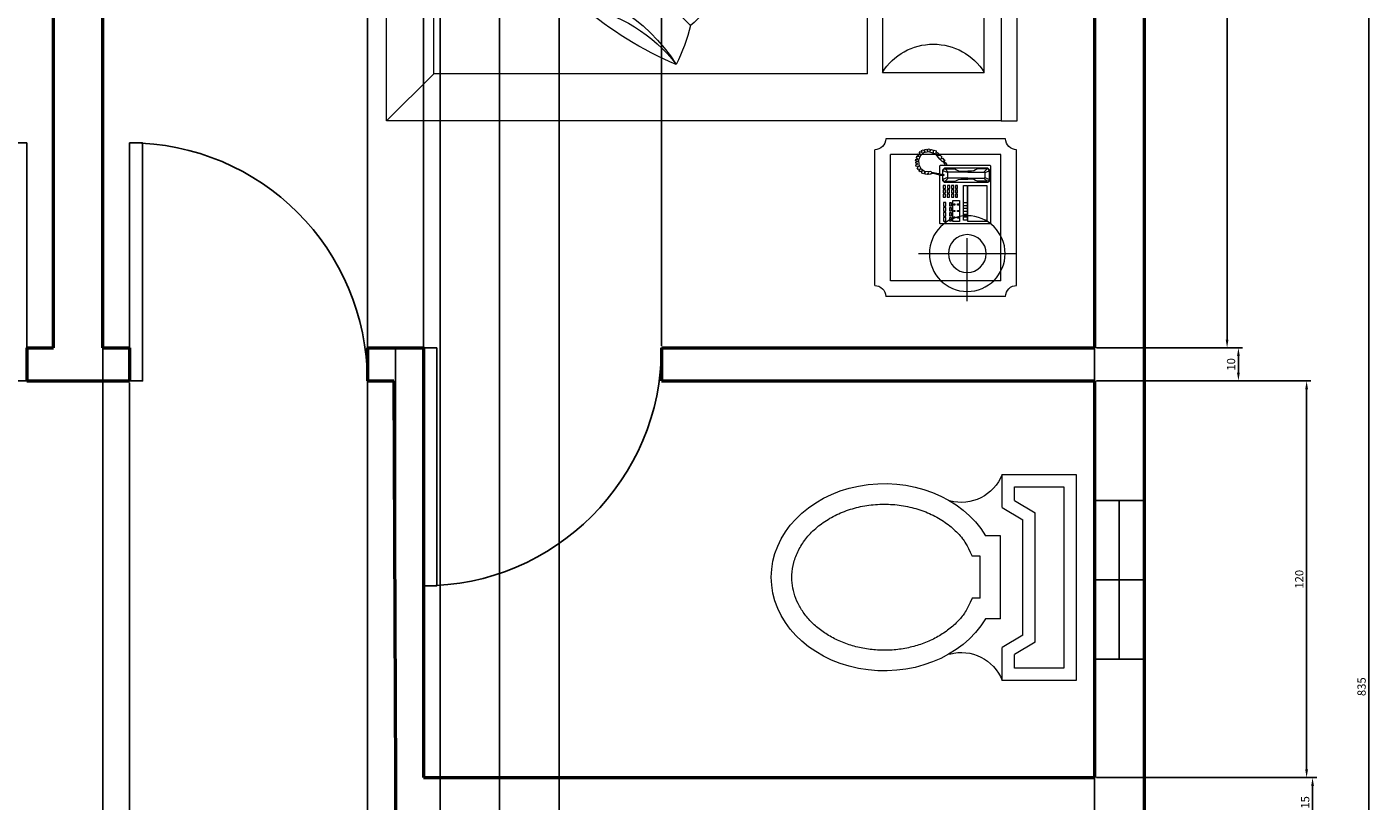
# Model space of a CAD drawing. Units: inches. Extents: x 604 to 3492, y -123 to 1737.
# Tile 16 of 20: x 1912 to 2319, y 836 to 1070. Entities that reach past the tile are written whole.
import ezdxf

# ---------------------------------------------------------------- set-up
doc = ezdxf.new("R2010")
doc.units = ezdxf.units.IN
for name, color, linetype, lineweight in [('A-ANNO-DIMS', 2, 'Continuous', 18), ('A-DOOR', 3, 'Continuous', 25), ('A-FLOR-FIXT', 9, 'Continuous', 18), ('A-FURN', 8, 'Continuous', 18), ('A-GLAZ', 4, 'Continuous', 25), ('A-WALL', 7, 'Continuous', 50)]:
    doc.layers.add(name, color=color, linetype=linetype, lineweight=lineweight)
doc.styles.get("Standard").update_dxf_attribs({"font": 'arial.ttf'})
doc.dimstyles.new('ISO-25', dxfattribs={"dimtxt": 2.5, "dimasz": 2.5, "dimexe": 1.25, "dimexo": 0.625, "dimtad": 1, "dimtxsty": 'Standard', "dimcen": 2.5, "dimadec": 0, "dimazin": 0, "dimtfac": 1, "dimtmove": 0, "dimatfit": 3, "dimfxl": 1, "dimarcsym": 0})

# ---------------------------------------------------------------- blocks, each defined once
blk = doc.blocks.new('A$C50B66110')
for p, q in [((0.0503, 1.9981), (0.4803, 1.9981)), ((0.1513, 1.6871), (0.1513, 1.9967)), ((0.5716, 1.9488), (0.5716, 2)), ((0.5716, 2), (2.0719, 2)), ((2.0719, 1.9488), (2.0719, 2)), ((2.1051, 1.9643), (2.1051, 1.5843)), ((2.5701, 1.9993), (2.1401, 1.9993)), ((2.6051, 1.9643), (2.6051, 1.5843)), ((0.0153, 1.9631), (0.0153, 1.5831)), ((0.0653, 1.9481), (0.0653, 1.5981)), ((0.0653, 1.9481), (0.4653, 1.9481)), ((0.4653, 1.9481), (0.4653, 1.5981)), ((0.5153, 1.9631), (0.5153, 1.5831)), ((2.0719, 1.9488), (0.5716, 1.9488)), ((0.5716, 1.9488), (0.5716, 0)), ((2.0719, 0), (2.0719, 1.9488)), ((2.1551, 1.9493), (2.1551, 1.5993)), ((2.5551, 1.9493), (2.1551, 1.9493)), ((2.3505, 1.62), (2.3505, 1.9295)), ((2.5551, 1.9493), (2.5551, 1.5993)), ((0.7257, 1.5725), (0.7257, 1.8954)), ((0.7257, 1.8954), (1.2113, 1.8954)), ((1.2113, 1.8954), (1.2113, 1.5725)), ((1.4007, 1.5725), (1.4007, 1.8954)), ((1.4007, 1.8954), (1.8863, 1.8954)), ((1.8863, 1.8954), (1.8863, 1.5725)), ((0, 1.8416), (0.2001, 1.8416)), ((2.5018, 1.7744), (2.2017, 1.7744)), ((0.0653, 1.5981), (0.4653, 1.5981)), ((2.5551, 1.5993), (2.1551, 1.5993)), ((0.0503, 1.5481), (0.4803, 1.5481)), ((1.2113, 1.5725), (0.7257, 1.5725)), ((1.8863, 1.5725), (1.4007, 1.5725)), ((2.5701, 1.5493), (2.1401, 1.5493)), ((1.5665, 1.5254), (1.5665, 1.0802)), ((1.5665, 1.5254), (1.9219, 1.0802)), ((1.9219, 1.0802), (1.5665, 1.0802)), ((0.5716, 0), (0.7216, 0.15)), ((2.0719, 0), (1.9219, 0.15)), ((0.5716, 0), (2.0719, 0))]:
    blk.add_line(p, q)
at = {"linetype": 'ByBlock'}
for p, q in [((0.2481, 1.9162), (0.2458, 1.9139)), ((0.2458, 1.9139), (0.2458, 1.7562)), ((0.2481, 1.9162), (0.4287, 1.9162)), ((0.2526, 1.9036), (0.2526, 1.8431)), ((0.3669, 1.9036), (0.2526, 1.9036)), ((0.3669, 1.8431), (0.3669, 1.9036)), ((0.3772, 1.9071), (0.3818, 1.9128)), ((0.3772, 1.7688), (0.3772, 1.9071)), ((0.3818, 1.9094), (0.3807, 1.9048)), ((0.3807, 1.9048), (0.3807, 1.8739)), ((0.3807, 1.9048), (0.3909, 1.8945)), ((0.3818, 1.9128), (0.4161, 1.9128)), ((0.3864, 1.9116), (0.3818, 1.9094)), ((0.3921, 1.8968), (0.3864, 1.9116)), ((0.3864, 1.9116), (0.4138, 1.9116)), ((0.3909, 1.8945), (0.3921, 1.8968)), ((0.3909, 1.8431), (0.3909, 1.8945)), ((0.4081, 1.8968), (0.3921, 1.8968)), ((0.4081, 1.8968), (0.4138, 1.9116)), ((0.4092, 1.8945), (0.4081, 1.8968)), ((0.4195, 1.9048), (0.4092, 1.8945)), ((0.4092, 1.8431), (0.4092, 1.8945)), ((0.4138, 1.9116), (0.4184, 1.9094)), ((0.4161, 1.9128), (0.4218, 1.9071)), ((0.4184, 1.9094), (0.4195, 1.9048)), ((0.4195, 1.9048), (0.4195, 1.8739)), ((0.4218, 1.9071), (0.4218, 1.7699)), ((0.4287, 1.9162), (0.4309, 1.9139)), ((0.4309, 1.9139), (0.4309, 1.7562)), ((0.2526, 1.8431), (0.3669, 1.8431)), ((0.2572, 1.8408), (0.2572, 1.8294)), ((0.3669, 1.8408), (0.2572, 1.8408)), ((0.2664, 1.8408), (0.2664, 1.8294)), ((0.2755, 1.8408), (0.2755, 1.8294)), ((0.2846, 1.8408), (0.2846, 1.8294)), ((0.2938, 1.8408), (0.2938, 1.8294)), ((0.3029, 1.8408), (0.3029, 1.8294)), ((0.3121, 1.8408), (0.3121, 1.8294)), ((0.3669, 1.8294), (0.3669, 1.8408)), ((0.3807, 1.8739), (0.3829, 1.8682)), ((0.3829, 1.8682), (0.3864, 1.8625)), ((0.3864, 1.8625), (0.3875, 1.8545)), ((0.3875, 1.8545), (0.3875, 1.8431)), ((0.3875, 1.8214), (0.3875, 1.8431)), ((0.3909, 1.8431), (0.3909, 1.7813)), ((0.4092, 1.8431), (0.4092, 1.7813)), ((0.4138, 1.8625), (0.4127, 1.8545)), ((0.4127, 1.8545), (0.4127, 1.8431)), ((0.4127, 1.8214), (0.4127, 1.8431)), ((0.4172, 1.8682), (0.4138, 1.8625)), ((0.4195, 1.8739), (0.4172, 1.8682)), ((0.3201, 1.8168), (0.2526, 1.8168)), ((0.2526, 1.8168), (0.2526, 1.7962)), ((0.2526, 1.7962), (0.3201, 1.7962)), ((0.2572, 1.8294), (0.3669, 1.8294)), ((0.2675, 1.8145), (0.2641, 1.8145)), ((0.2641, 1.8145), (0.2641, 1.8111)), ((0.2641, 1.8111), (0.2675, 1.8111)), ((0.2641, 1.8019), (0.2641, 1.7985)), ((0.2675, 1.8019), (0.2641, 1.8019)), ((0.2641, 1.7985), (0.2675, 1.7985)), ((0.2675, 1.8111), (0.2675, 1.8145)), ((0.2675, 1.7985), (0.2675, 1.8019)), ((0.2846, 1.8145), (0.2846, 1.8111)), ((0.2881, 1.8145), (0.2846, 1.8145)), ((0.2846, 1.8111), (0.2881, 1.8111)), ((0.2846, 1.8019), (0.2846, 1.7985)), ((0.2881, 1.8019), (0.2846, 1.8019)), ((0.2846, 1.7985), (0.2881, 1.7985)), ((0.2881, 1.8111), (0.2881, 1.8145)), ((0.2881, 1.7985), (0.2881, 1.8019)), ((0.3052, 1.8145), (0.3052, 1.8111)), ((0.3086, 1.8145), (0.3052, 1.8145)), ((0.3052, 1.8111), (0.3086, 1.8111)), ((0.3052, 1.8019), (0.3052, 1.7985)), ((0.3086, 1.8019), (0.3052, 1.8019)), ((0.3052, 1.7985), (0.3086, 1.7985)), ((0.3086, 1.8111), (0.3086, 1.8145)), ((0.3086, 1.7985), (0.3086, 1.8019)), ((0.3201, 1.7962), (0.3201, 1.8168)), ((0.3304, 1.8111), (0.3395, 1.8111)), ((0.3304, 1.8042), (0.3304, 1.8111)), ((0.3395, 1.8042), (0.3304, 1.8042)), ((0.3304, 1.7985), (0.3395, 1.7985)), ((0.3304, 1.7916), (0.3304, 1.7985)), ((0.3395, 1.8111), (0.3395, 1.8042)), ((0.3395, 1.7985), (0.3395, 1.7916)), ((0.3441, 1.8042), (0.3441, 1.8111)), ((0.3441, 1.8111), (0.3532, 1.8111)), ((0.3532, 1.8042), (0.3441, 1.8042)), ((0.3441, 1.7985), (0.3532, 1.7985)), ((0.3441, 1.7916), (0.3441, 1.7985)), ((0.3532, 1.8111), (0.3532, 1.8042)), ((0.3532, 1.7985), (0.3532, 1.7916)), ((0.3578, 1.8111), (0.3669, 1.8111)), ((0.3578, 1.8042), (0.3578, 1.8111)), ((0.3669, 1.8042), (0.3578, 1.8042)), ((0.3578, 1.7985), (0.3669, 1.7985)), ((0.3578, 1.7916), (0.3578, 1.7985)), ((0.3669, 1.8111), (0.3669, 1.8042)), ((0.3669, 1.7985), (0.3669, 1.7916)), ((0.3807, 1.8019), (0.3829, 1.8076)), ((0.3807, 1.7711), (0.3807, 1.8019)), ((0.3829, 1.8076), (0.3864, 1.8134)), ((0.3864, 1.8134), (0.3875, 1.8214)), ((0.4138, 1.8134), (0.4127, 1.8214)), ((0.4172, 1.8076), (0.4138, 1.8134)), ((0.4195, 1.8019), (0.4172, 1.8076)), ((0.4195, 1.7711), (0.4195, 1.8019)), ((0.2458, 1.7562), (0.2481, 1.7539)), ((0.4, 1.7539), (0.2481, 1.7539)), ((0.2652, 1.7905), (0.2538, 1.7905)), ((0.2538, 1.7905), (0.2538, 1.7859)), ((0.2538, 1.7859), (0.2652, 1.7859)), ((0.2538, 1.7665), (0.2538, 1.7733)), ((0.2538, 1.7733), (0.2652, 1.7733)), ((0.2652, 1.7665), (0.2538, 1.7665)), ((0.2652, 1.7859), (0.2652, 1.7905)), ((0.2652, 1.7733), (0.2652, 1.7665)), ((0.2812, 1.7905), (0.2698, 1.7905)), ((0.2698, 1.7905), (0.2698, 1.7859)), ((0.2698, 1.7859), (0.2812, 1.7859)), ((0.2698, 1.7665), (0.2698, 1.7733)), ((0.2698, 1.7733), (0.2812, 1.7733)), ((0.2812, 1.7665), (0.2698, 1.7665)), ((0.2812, 1.7859), (0.2812, 1.7905)), ((0.2812, 1.7733), (0.2812, 1.7665)), ((0.2972, 1.7905), (0.2858, 1.7905)), ((0.2858, 1.7905), (0.2858, 1.7859)), ((0.2858, 1.7859), (0.2972, 1.7859)), ((0.2858, 1.7665), (0.2858, 1.7733)), ((0.2858, 1.7733), (0.2972, 1.7733)), ((0.2972, 1.7665), (0.2858, 1.7665)), ((0.2972, 1.7859), (0.2972, 1.7905)), ((0.2972, 1.7733), (0.2972, 1.7665)), ((0.3018, 1.7905), (0.3018, 1.7859)), ((0.3132, 1.7905), (0.3018, 1.7905)), ((0.3018, 1.7859), (0.3132, 1.7859)), ((0.3018, 1.7733), (0.3132, 1.7733)), ((0.3018, 1.7665), (0.3018, 1.7733)), ((0.3132, 1.7665), (0.3018, 1.7665)), ((0.3132, 1.7859), (0.3132, 1.7905)), ((0.3132, 1.7733), (0.3132, 1.7665)), ((0.3395, 1.7916), (0.3304, 1.7916)), ((0.3304, 1.7779), (0.3304, 1.7848)), ((0.3304, 1.7848), (0.3395, 1.7848)), ((0.3395, 1.7779), (0.3304, 1.7779)), ((0.3304, 1.7722), (0.3395, 1.7722)), ((0.3304, 1.7653), (0.3304, 1.7722)), ((0.3395, 1.7653), (0.3304, 1.7653)), ((0.3395, 1.7848), (0.3395, 1.7779)), ((0.3395, 1.7722), (0.3395, 1.7653)), ((0.3532, 1.7916), (0.3441, 1.7916)), ((0.3441, 1.7779), (0.3441, 1.7848)), ((0.3441, 1.7848), (0.3532, 1.7848)), ((0.3532, 1.7779), (0.3441, 1.7779)), ((0.3441, 1.7722), (0.3532, 1.7722)), ((0.3441, 1.7653), (0.3441, 1.7722)), ((0.3532, 1.7653), (0.3441, 1.7653)), ((0.3532, 1.7848), (0.3532, 1.7779)), ((0.3532, 1.7722), (0.3532, 1.7653)), ((0.3669, 1.7916), (0.3578, 1.7916)), ((0.3578, 1.7791), (0.3578, 1.7859)), ((0.3578, 1.7859), (0.3669, 1.7859)), ((0.3669, 1.7791), (0.3578, 1.7791)), ((0.3578, 1.7653), (0.3578, 1.7722)), ((0.3578, 1.7722), (0.3669, 1.7722)), ((0.3669, 1.7653), (0.3578, 1.7653)), ((0.3669, 1.7859), (0.3669, 1.7791)), ((0.3669, 1.7722), (0.3669, 1.7653)), ((0.3829, 1.7631), (0.3772, 1.7688)), ((0.3807, 1.7711), (0.3909, 1.7813)), ((0.3818, 1.7665), (0.3807, 1.7711)), ((0.3864, 1.7642), (0.3818, 1.7665)), ((0.399, 1.7631), (0.3829, 1.7631)), ((0.3921, 1.7791), (0.3864, 1.7642)), ((0.3864, 1.7642), (0.399, 1.7642)), ((0.3909, 1.7813), (0.3921, 1.7791)), ((0.4081, 1.7791), (0.3921, 1.7791)), ((0.4024, 1.7676), (0.3989, 1.7676)), ((0.3989, 1.7676), (0.3991, 1.7578)), ((0.3991, 1.7578), (0.4019, 1.7462)), ((0.403, 1.7585), (0.4024, 1.7676)), ((0.4026, 1.7642), (0.4138, 1.7642)), ((0.4161, 1.7631), (0.4027, 1.7631)), ((0.4047, 1.7511), (0.403, 1.7585)), ((0.4287, 1.7539), (0.404, 1.7539)), ((0.4074, 1.7402), (0.4047, 1.7511)), ((0.4092, 1.7813), (0.4081, 1.7791)), ((0.4081, 1.7791), (0.4138, 1.7642)), ((0.4195, 1.7711), (0.4092, 1.7813)), ((0.4138, 1.7642), (0.4184, 1.7665)), ((0.4218, 1.7699), (0.4161, 1.7631)), ((0.4184, 1.7665), (0.4195, 1.7711)), ((0.4309, 1.7562), (0.4287, 1.7539)), ((0.4378, 1.7742), (0.4309, 1.7768)), ((0.4309, 1.7722), (0.436, 1.7708)), ((0.436, 1.7708), (0.4406, 1.7672)), ((0.441, 1.771), (0.4378, 1.7742)), ((0.4406, 1.7672), (0.4418, 1.7656)), ((0.4434, 1.7688), (0.441, 1.771)), ((0.4443, 1.7658), (0.4418, 1.7633)), ((0.4418, 1.7656), (0.4443, 1.7658)), ((0.4418, 1.7633), (0.4511, 1.7551)), ((0.4477, 1.7704), (0.4434, 1.7688)), ((0.4497, 1.7684), (0.4477, 1.7704)), ((0.4481, 1.765), (0.4497, 1.7684)), ((0.4509, 1.7672), (0.4481, 1.765)), ((0.4539, 1.764), (0.4509, 1.7672)), ((0.4511, 1.7551), (0.4662, 1.7422)), ((0.4515, 1.7573), (0.4539, 1.764)), ((0.4577, 1.7605), (0.4515, 1.7573)), ((0.463, 1.7555), (0.4577, 1.7605)), ((0.4618, 1.7482), (0.463, 1.7555)), ((0.467, 1.7515), (0.4618, 1.7482)), ((0.4714, 1.7468), (0.467, 1.7515)), ((0.4019, 1.7462), (0.4047, 1.7353)), ((0.4026, 1.7254), (0.4021, 1.7198)), ((0.4021, 1.7198), (0.4088, 1.7187)), ((0.4088, 1.7187), (0.4023, 1.7147)), ((0.4023, 1.7147), (0.4028, 1.7085)), ((0.4051, 1.7279), (0.4026, 1.7254)), ((0.4028, 1.7085), (0.4102, 1.7078)), ((0.4102, 1.7078), (0.4037, 1.7027)), ((0.4047, 1.7353), (0.4044, 1.7293)), ((0.4044, 1.7293), (0.4051, 1.7279)), ((0.4081, 1.7346), (0.4074, 1.7402)), ((0.4079, 1.7286), (0.4081, 1.7346)), ((0.4121, 1.7256), (0.4079, 1.7286)), ((0.4111, 1.7203), (0.4121, 1.7256)), ((0.4123, 1.7057), (0.4111, 1.7203)), ((0.4664, 1.7418), (0.4741, 1.72)), ((0.4696, 1.7418), (0.4714, 1.7468)), ((0.4766, 1.7425), (0.4697, 1.7418)), ((0.4741, 1.72), (0.4708, 1.7027)), ((0.472, 1.733), (0.4787, 1.7356)), ((0.4794, 1.7332), (0.472, 1.733)), ((0.4743, 1.7075), (0.4815, 1.7073)), ((0.4798, 1.7013), (0.4743, 1.7075)), ((0.4761, 1.7233), (0.481, 1.7279)), ((0.4824, 1.7233), (0.4761, 1.7233)), ((0.4764, 1.7154), (0.4835, 1.7175)), ((0.4824, 1.7119), (0.4764, 1.7154)), ((0.4787, 1.7356), (0.4766, 1.7425)), ((0.481, 1.7279), (0.4794, 1.7332)), ((0.4815, 1.7073), (0.4824, 1.7119)), ((0.4835, 1.7175), (0.4824, 1.7233)), ((0.4037, 1.7027), (0.4067, 1.6974)), ((0.4067, 1.6974), (0.4137, 1.6988)), ((0.4137, 1.6988), (0.4104, 1.6923)), ((0.4104, 1.6923), (0.4139, 1.6881)), ((0.4211, 1.6946), (0.4123, 1.7057)), ((0.4139, 1.6881), (0.4192, 1.692)), ((0.4192, 1.692), (0.4183, 1.6858)), ((0.4183, 1.6858), (0.4227, 1.683)), ((0.4333, 1.6881), (0.4211, 1.6946)), ((0.4227, 1.683), (0.4283, 1.6876)), ((0.4283, 1.6876), (0.4276, 1.68)), ((0.4276, 1.68), (0.4324, 1.6786)), ((0.4324, 1.6786), (0.4354, 1.6849)), ((0.4472, 1.6869), (0.4333, 1.6881)), ((0.4354, 1.6849), (0.4382, 1.6786)), ((0.4382, 1.6786), (0.4421, 1.6782)), ((0.4421, 1.6782), (0.4437, 1.6849)), ((0.4437, 1.6849), (0.4463, 1.6775)), ((0.4463, 1.6775), (0.4507, 1.6786)), ((0.4606, 1.6927), (0.4472, 1.6869)), ((0.4507, 1.6786), (0.4509, 1.6849)), ((0.4509, 1.6849), (0.4562, 1.6802)), ((0.4562, 1.6802), (0.4599, 1.6821)), ((0.4592, 1.689), (0.4641, 1.683)), ((0.4599, 1.6821), (0.4592, 1.689)), ((0.4708, 1.7027), (0.4606, 1.6927)), ((0.4641, 1.683), (0.4678, 1.6863)), ((0.465, 1.6925), (0.4715, 1.6897)), ((0.4678, 1.6863), (0.465, 1.6925)), ((0.4745, 1.6925), (0.4713, 1.6988)), ((0.4713, 1.6988), (0.478, 1.6967)), ((0.4715, 1.6897), (0.4745, 1.6925)), ((0.478, 1.6967), (0.4798, 1.7013)), ((0.7216, 1.5254), (1.9219, 1.5254)), ((0.7216, 1.5254), (0.7216, 0.15)), ((1.9219, 0.15), (1.9219, 1.5254)), ((0.7216, 0.15), (1.9219, 0.15))]:
    blk.add_line(p, q, dxfattribs=at)
for centre, radius in [((0.1513, 1.8416), 0.12), ((0.1513, 1.8416), 0.06), ((2.3505, 1.7744), 0.12), ((2.3505, 1.7744), 0.06)]:
    blk.add_circle(centre, radius)
for centre, radius, start, end in [((0.0153, 1.9981), 0.035, 270, 0), ((0.5153, 1.9981), 0.035, 180, 270), ((2.1051, 1.9993), 0.035, 270, 0), ((2.6051, 1.9993), 0.035, 180, 270), ((0.6244, 1.734), 0.1906, 302.1202, 57.8798), ((1.3126, 1.734), 0.1906, 122.1202, 237.8798), ((1.2994, 1.734), 0.1906, 302.1202, 57.8798), ((1.9876, 1.734), 0.1906, 122.1202, 237.8798), ((0.0153, 1.5481), 0.035, 0, 90), ((0.5153, 1.5481), 0.035, 90, 180), ((2.1051, 1.5493), 0.035, 0, 90), ((2.6051, 1.5493), 0.035, 90, 180), ((1.1502, 0.7366), 0.3575, 102.4782, 140.4625), ((0.328, 0.4368), 0.9879, 28.4971, 41.0566), ((1.9117, 1.3157), 0.8697, 195.336, 226.4193), ((0.9996, 0.4307), 0.548, 103.2034, 117.0362), ((1.656, 1.7093), 1.0798, 223.6306, 251.4288), ((0.4482, 0.4408), 0.5655, 5.3391, 57.6895), ((1.8226, 1.3753), 1.1652, 203.0642, 220.3209), ((0.4548, 0.5307), 0.4879, 10.6986, 52.6864), ((0.5648, 0.4378), 0.7874, 18.3527, 36.6851), ((-0.0179, 2.4352), 2.1977, 305.2966, 307.2418), ((1.4166, 0.4903), 0.3575, 154.0418, 192.0262), ((1.1403, -0.3401), 0.9879, 80.0607, 92.6202), ((1.5981, 0.9345), 0.734, 205.259, 216.9351), ((1.3672, 0.0075), 0.6085, 71.81, 120.1351), ((1.4431, 0.1219), 0.4774, 76.1849, 142.0017), ((1.2867, -0.154), 0.7874, 69.9163, 88.2487), ((-0.6401, 0.6314), 2.1977, 349.4884, 358.8054), ((-0.0179, 2.4352), 2.1977, 297.9248, 299.3793), ((1.5626, 0.1822), 0.548, 154.767, 168.5998), ((1.2678, 0.9611), 0.6885, 250.2936, 293.6414), ((1.3343, 1.4141), 1.1652, 254.6278, 271.8845), ((1.5399, 0.9642), 0.734, 256.8226, 268.4988)]:
    blk.add_arc(centre, radius, start, end)
blk = doc.blocks.new('A$C7C8779AE')
for p, q in [((0, 0.7405), (0, 0.5605)), ((0.5, 0.7405), (0, 0.7405)), ((0.5, 0.5605), (0.5, 0.7405)), ((0.47, 0.7105), (0.03, 0.7105)), ((0.03, 0.7105), (0.03, 0.5905)), ((0.47, 0.5905), (0.47, 0.7105)), ((0.093, 0.6405), (0.063, 0.5905)), ((0.093, 0.6405), (0.407, 0.6405)), ((0.437, 0.5905), (0.407, 0.6405)), ((0.03, 0.5905), (0.063, 0.5905)), ((0.11, 0.6105), (0.08, 0.5605)), ((0.11, 0.6105), (0.39, 0.6105)), ((0.42, 0.5605), (0.39, 0.6105)), ((0.437, 0.5905), (0.47, 0.5905)), ((0, 0.5605), (0.08, 0.5605)), ((0.1497, 0.557), (0.1497, 0.5203)), ((0.1497, 0.557), (0.3514, 0.557)), ((0.3514, 0.557), (0.3514, 0.5203)), ((0.42, 0.5605), (0.5, 0.5605)), ((0.1997, 0.507), (0.1997, 0.4879)), ((0.1997, 0.507), (0.3014, 0.507)), ((0.3014, 0.507), (0.3014, 0.4879))]:
    blk.add_line(p, q)
for centre, start, end in [((-0.0386, 0.4613), 344.642, 68.7339), ((0.5386, 0.4613), 111.2661, 195.358)]:
    blk.add_arc(centre, 0.1064, start, end)
blk.add_ellipse((0.2506, 0.2744), major_axis=(0, 0.2744), ratio=0.828948, start_param=0.459479, end_param=5.823706)
blk.add_open_spline([(0.1997, 0.4879), (0.1697, 0.474), (0.1642, 0.4702), (0.1512, 0.4602), (0.1438, 0.4535), (0.1298, 0.4388), (0.1233, 0.4306), (0.1111, 0.4131), (0.1055, 0.4037), (0.0956, 0.3838), (0.0912, 0.3733), (0.0838, 0.3516), (0.0808, 0.3403), (0.0762, 0.3172), (0.0746, 0.3055), (0.073, 0.2817), (0.0729, 0.2698), (0.0743, 0.246), (0.0758, 0.2342), (0.0801, 0.2111), (0.0831, 0.1998), (0.0903, 0.1779), (0.0945, 0.1673), (0.1043, 0.1473), (0.1098, 0.1378), (0.1218, 0.12), (0.1283, 0.1118), (0.1421, 0.0968), (0.1494, 0.09), (0.1646, 0.078), (0.1725, 0.0728), (0.1887, 0.064), (0.1969, 0.0603), (0.2137, 0.0547), (0.2222, 0.0527), (0.2392, 0.0502), (0.2478, 0.0498), (0.2664, 0.0505), (0.2764, 0.052), (0.2963, 0.0573), (0.3061, 0.061), (0.3253, 0.0707), (0.3346, 0.0766), (0.3525, 0.0906), (0.3611, 0.0987), (0.3771, 0.1169), (0.3845, 0.127), (0.3978, 0.1488), (0.4037, 0.1605), (0.4137, 0.1853), (0.4178, 0.1983), (0.424, 0.2251), (0.4261, 0.2389), (0.4282, 0.2668), (0.4283, 0.2809), (0.4262, 0.3088), (0.4241, 0.3226), (0.418, 0.3495), (0.414, 0.3625), (0.404, 0.3873), (0.3982, 0.3991), (0.385, 0.421), (0.3776, 0.4311), (0.3617, 0.4494), (0.3531, 0.4575), (0.3382, 0.4693), (0.3321, 0.4736), (0.3014, 0.4879)], degree=3, knots=[0.459479, 0.459479, 0.459479, 0.459479, 0.567422, 0.567422, 0.720865, 0.720865, 0.874307, 0.874307, 1.02775, 1.02775, 1.181192, 1.181192, 1.334635, 1.334635, 1.488077, 1.488077, 1.64152, 1.64152, 1.794963, 1.794963, 1.948405, 1.948405, 2.101848, 2.101848, 2.25529, 2.25529, 2.408733, 2.408733, 2.562175, 2.562175, 2.715618, 2.715618, 2.86906, 2.86906, 3.022503, 3.022503, 3.175946, 3.175946, 3.356457, 3.356457, 3.536968, 3.536968, 3.717479, 3.717479, 3.89799, 3.89799, 4.078501, 4.078501, 4.259012, 4.259012, 4.439523, 4.439523, 4.620035, 4.620035, 4.800546, 4.800546, 4.981057, 4.981057, 5.161568, 5.161568, 5.342079, 5.342079, 5.52259, 5.52259, 5.703101, 5.703101, 5.823706, 5.823706, 5.823706, 5.823706])
blk = doc.blocks.new('*D44')
at = {"layer": 'A-ANNO-DIMS', "color": 0, "lineweight": -2, "transparency": 16777216}
for p, q in [((2235.2, 1272.7), (2275.95, 1272.7)), ((2274.7, 975.2), (2274.7, 1270.2)), ((2235.2, 972.7), (2275.95, 972.7))]:
    blk.add_line(p, q, dxfattribs=at)
at = {"layer": 'A-ANNO-DIMS', "color": 0, "transparency": 16777216}
for points in [[(2274.28, 1270.2), (2275.11, 1270.2), (2274.7, 1272.7)], [(2274.28, 975.2), (2275.11, 975.2), (2274.7, 972.7)]]:
    blk.add_solid(points, dxfattribs=at)
at = {"layer": 'Defpoints', "color": 0, "transparency": 16777216}
for p in [(2234.57, 1272.7), (2274.7, 1272.7), (2234.57, 972.7)]:
    blk.add_point(p, dxfattribs=at)
at = {"layer": 'A-ANNO-DIMS', "color": 0, "transparency": 16777216, "insert": (2272.79, 1122.7), "char_height": 2.5, "attachment_point": 5, "rotation": 90}
blk.add_mtext('300', dxfattribs=at)
blk = doc.blocks.new('*D45')
at = {"layer": 'A-ANNO-DIMS', "color": 0, "lineweight": -2, "transparency": 16777216}
for p, q in [((2235.2, 972.7), (2279.37, 972.7)), ((2278.12, 970.2), (2278.12, 965.2)), ((2235.2, 962.7), (2279.37, 962.7))]:
    blk.add_line(p, q, dxfattribs=at)
at = {"layer": 'A-ANNO-DIMS', "color": 0, "transparency": 16777216}
for points in [[(2277.7, 970.2), (2278.54, 970.2), (2278.12, 972.7)], [(2277.7, 965.2), (2278.54, 965.2), (2278.12, 962.7)]]:
    blk.add_solid(points, dxfattribs=at)
at = {"layer": 'Defpoints', "color": 0, "transparency": 16777216}
for p in [(2234.57, 972.7), (2234.57, 962.7), (2278.12, 962.7)]:
    blk.add_point(p, dxfattribs=at)
at = {"layer": 'A-ANNO-DIMS', "color": 0, "transparency": 16777216, "insert": (2276.22, 967.7), "char_height": 2.5, "attachment_point": 5, "rotation": 90}
blk.add_mtext('10', dxfattribs=at)
blk = doc.blocks.new('*D46')
at = {"layer": 'A-ANNO-DIMS', "color": 0, "lineweight": -2, "transparency": 16777216}
for p, q in [((2235.2, 962.7), (2300, 962.7)), ((2298.75, 960.2), (2298.75, 845.2)), ((2235.2, 842.7), (2300, 842.7))]:
    blk.add_line(p, q, dxfattribs=at)
at = {"layer": 'A-ANNO-DIMS', "color": 0, "transparency": 16777216}
for points in [[(2298.34, 960.2), (2299.17, 960.2), (2298.75, 962.7)], [(2298.34, 845.2), (2299.17, 845.2), (2298.75, 842.7)]]:
    blk.add_solid(points, dxfattribs=at)
at = {"layer": 'Defpoints', "color": 0, "transparency": 16777216}
for p in [(2234.57, 962.7), (2234.57, 842.7), (2298.75, 842.7)]:
    blk.add_point(p, dxfattribs=at)
at = {"layer": 'A-ANNO-DIMS', "color": 0, "transparency": 16777216, "insert": (2296.85, 902.7), "char_height": 2.5, "attachment_point": 5, "rotation": 90}
blk.add_mtext('120', dxfattribs=at)
blk = doc.blocks.new('*D47')
at = {"layer": 'A-ANNO-DIMS', "color": 0, "lineweight": -2, "transparency": 16777216}
for p, q in [((2235.2, 842.7), (2301.8, 842.7)), ((2300.55, 840.2), (2300.55, 830.2)), ((2235.2, 827.7), (2301.8, 827.7))]:
    blk.add_line(p, q, dxfattribs=at)
at = {"layer": 'A-ANNO-DIMS', "color": 0, "transparency": 16777216}
for points in [[(2300.13, 840.2), (2300.96, 840.2), (2300.55, 842.7)], [(2300.13, 830.2), (2300.96, 830.2), (2300.55, 827.7)]]:
    blk.add_solid(points, dxfattribs=at)
at = {"layer": 'Defpoints', "color": 0, "transparency": 16777216}
for p in [(2234.57, 842.7), (2234.57, 827.7), (2300.55, 827.7)]:
    blk.add_point(p, dxfattribs=at)
at = {"layer": 'A-ANNO-DIMS', "color": 0, "transparency": 16777216, "insert": (2298.64, 835.2), "char_height": 2.5, "attachment_point": 5, "rotation": 90}
blk.add_mtext('15', dxfattribs=at)
blk = doc.blocks.new('*D70')
at = {"layer": 'A-ANNO-DIMS', "color": 0, "lineweight": -2, "transparency": 16777216}
for p, q in [((2250.2, 1287.7), (2318.86, 1287.7)), ((2317.61, 455.2), (2317.61, 1285.2)), ((2250.2, 452.7), (2318.86, 452.7))]:
    blk.add_line(p, q, dxfattribs=at)
at = {"layer": 'A-ANNO-DIMS', "color": 0, "transparency": 16777216}
for points in [[(2317.2, 1285.2), (2318.03, 1285.2), (2317.61, 1287.7)], [(2317.2, 455.2), (2318.03, 455.2), (2317.61, 452.7)]]:
    blk.add_solid(points, dxfattribs=at)
at = {"layer": 'Defpoints', "color": 0, "transparency": 16777216}
for p in [(2249.57, 1287.7), (2317.61, 1287.7), (2249.57, 452.7)]:
    blk.add_point(p, dxfattribs=at)
at = {"layer": 'A-ANNO-DIMS', "color": 0, "transparency": 16777216, "insert": (2315.71, 870.2), "char_height": 2.5, "attachment_point": 5, "rotation": 90}
blk.add_mtext('835', dxfattribs=at)
blk = doc.blocks.new('DOOR-SWING-72')
for p, q in [((0, 72), (0, 0)), ((0, 0), (4, 0)), ((0, 0), (4, 0))]:
    blk.add_line(p, q)
blk.add_lwpolyline([(0, 72), (0, 0), (4, 0), (4, 72)], close=True)
blk.add_arc((0, 0), 72, 0, 90)
blk = doc.blocks.new('WIN-48')
for p, q in [((0, 48), (15, 48)), ((7.5, 48), (7.5, 0)), ((15, 48), (15, 0)), ((0, 24), (15, 24))]:
    blk.add_line(p, q)
blk.add_lwpolyline([(15, 0), (0, 0), (0, 48), (15, 48)], close=True)
blk = doc.blocks.new('*D101')
at = {"layer": 'A-ANNO-DIMS', "color": 0, "lineweight": -2, "transparency": 16777216}
for p, q in [((2031.57, 843.33), (2031.57, 1359.9)), ((2034.07, 1358.65), (2232.07, 1358.65)), ((2234.57, 843.33), (2234.57, 1359.9))]:
    blk.add_line(p, q, dxfattribs=at)
at = {"layer": 'A-ANNO-DIMS', "color": 0, "transparency": 16777216}
for points in [[(2034.07, 1359.07), (2034.07, 1358.23), (2031.57, 1358.65)], [(2232.07, 1359.07), (2232.07, 1358.23), (2234.57, 1358.65)]]:
    blk.add_solid(points, dxfattribs=at)
at = {"layer": 'Defpoints', "color": 0, "transparency": 16777216}
for p in [(2234.57, 1358.65), (2031.57, 842.7), (2234.57, 842.7)]:
    blk.add_point(p, dxfattribs=at)
at = {"layer": 'A-ANNO-DIMS', "color": 0, "transparency": 16777216, "insert": (2133.07, 1360.55), "char_height": 2.5, "attachment_point": 5}
blk.add_mtext('203', dxfattribs=at)
blk = doc.blocks.new('*D102')
at = {"layer": 'A-ANNO-DIMS', "color": 0, "lineweight": -2, "transparency": 16777216}
for p, q in [((1839.57, 972.08), (1839.57, 215.5)), ((2023.07, 972.08), (2023.07, 215.5)), ((1842.07, 216.75), (2020.57, 216.75))]:
    blk.add_line(p, q, dxfattribs=at)
at = {"layer": 'A-ANNO-DIMS', "color": 0, "transparency": 16777216}
for points in [[(1842.07, 217.17), (1842.07, 216.33), (1839.57, 216.75)], [(2020.57, 217.17), (2020.57, 216.33), (2023.07, 216.75)]]:
    blk.add_solid(points, dxfattribs=at)
at = {"layer": 'Defpoints', "color": 0, "transparency": 16777216}
for p in [(1839.57, 972.7), (2023.07, 972.7), (2023.07, 216.75)]:
    blk.add_point(p, dxfattribs=at)
at = {"layer": 'A-ANNO-DIMS', "color": 0, "transparency": 16777216, "insert": (1931.32, 218.65), "char_height": 2.5, "attachment_point": 5}
blk.add_mtext('183.5', dxfattribs=at)
blk = doc.blocks.new('*D104')
at = {"layer": 'A-ANNO-DIMS', "color": 0, "lineweight": -2, "transparency": 16777216}
for p, q in [((1934.57, 1272.08), (1934.57, 215.5)), ((2036.57, 1272.08), (2036.57, 215.5)), ((1937.07, 216.75), (2034.07, 216.75))]:
    blk.add_line(p, q, dxfattribs=at)
at = {"layer": 'A-ANNO-DIMS', "color": 0, "transparency": 16777216}
for points in [[(1937.07, 217.17), (1937.07, 216.33), (1934.57, 216.75)], [(2034.07, 217.17), (2034.07, 216.33), (2036.57, 216.75)]]:
    blk.add_solid(points, dxfattribs=at)
at = {"layer": 'Defpoints', "color": 0, "transparency": 16777216}
for p in [(1934.57, 1272.7), (2036.57, 1272.7), (2036.57, 216.75)]:
    blk.add_point(p, dxfattribs=at)
at = {"layer": 'A-ANNO-DIMS', "color": 0, "transparency": 16777216, "insert": (1985.57, 218.65), "char_height": 2.5, "attachment_point": 5}
blk.add_mtext('102', dxfattribs=at)
blk = doc.blocks.new('*D109')
at = {"layer": 'A-ANNO-DIMS', "color": 0, "lineweight": -2, "transparency": 16777216}
for p, q in [((2054.57, 740.33), (2054.57, 1359.9)), ((2057.07, 1358.65), (2232.07, 1358.65)), ((2234.57, 740.33), (2234.57, 1359.9))]:
    blk.add_line(p, q, dxfattribs=at)
at = {"layer": 'A-ANNO-DIMS', "color": 0, "transparency": 16777216}
for points in [[(2057.07, 1359.07), (2057.07, 1358.23), (2054.57, 1358.65)], [(2232.07, 1359.07), (2232.07, 1358.23), (2234.57, 1358.65)]]:
    blk.add_solid(points, dxfattribs=at)
at = {"layer": 'Defpoints', "color": 0, "transparency": 16777216}
for p in [(2234.57, 1358.65), (2054.57, 739.7), (2234.57, 739.7)]:
    blk.add_point(p, dxfattribs=at)
at = {"layer": 'A-ANNO-DIMS', "color": 0, "transparency": 16777216, "insert": (2144.57, 1360.55), "char_height": 2.5, "attachment_point": 5}
blk.add_mtext('180', dxfattribs=at)
blk = doc.blocks.new('*D111')
at = {"layer": 'A-ANNO-DIMS', "color": 0, "lineweight": -2, "transparency": 16777216}
for p, q in [((2103.57, 973.33), (2103.57, 1359.9)), ((2106.07, 1358.65), (2232.07, 1358.65)), ((2234.57, 973.33), (2234.57, 1359.9))]:
    blk.add_line(p, q, dxfattribs=at)
at = {"layer": 'A-ANNO-DIMS', "color": 0, "transparency": 16777216}
for points in [[(2106.07, 1359.07), (2106.07, 1358.23), (2103.57, 1358.65)], [(2232.07, 1359.07), (2232.07, 1358.23), (2234.57, 1358.65)]]:
    blk.add_solid(points, dxfattribs=at)
at = {"layer": 'Defpoints', "color": 0, "transparency": 16777216}
for p in [(2234.57, 1358.65), (2103.57, 972.7), (2234.57, 972.7)]:
    blk.add_point(p, dxfattribs=at)
at = {"layer": 'A-ANNO-DIMS', "color": 0, "transparency": 16777216, "insert": (2169.07, 1360.55), "char_height": 2.5, "attachment_point": 5}
blk.add_mtext('131', dxfattribs=at)
blk = doc.blocks.new('*D112')
at = {"layer": 'A-ANNO-DIMS', "color": 0, "lineweight": -2, "transparency": 16777216}
for p, q in [((1934.57, 972.08), (1934.57, 215.5)), ((1942.57, 962.08), (1942.57, 215.5)), ((1940.07, 216.75), (1937.07, 216.75))]:
    blk.add_line(p, q, dxfattribs=at)
at = {"layer": 'A-ANNO-DIMS', "color": 0, "transparency": 16777216}
for points in [[(1937.07, 217.17), (1937.07, 216.33), (1934.57, 216.75)], [(1940.07, 217.17), (1940.07, 216.33), (1942.57, 216.75)]]:
    blk.add_solid(points, dxfattribs=at)
at = {"layer": 'Defpoints', "color": 0, "transparency": 16777216}
for p in [(1934.57, 972.7), (1942.57, 962.7), (1934.57, 216.75)]:
    blk.add_point(p, dxfattribs=at)
at = {"layer": 'A-ANNO-DIMS', "color": 0, "transparency": 16777216, "insert": (1938.57, 218.65), "char_height": 2.5, "attachment_point": 5}
blk.add_mtext('8', dxfattribs=at)
blk = doc.blocks.new('*D113')
at = {"layer": 'A-ANNO-DIMS', "color": 0, "lineweight": -2, "transparency": 16777216}
for p, q in [((2014.57, 603.33), (2014.57, 1359.9)), ((2017.07, 1358.65), (2070.07, 1358.65)), ((2072.57, 603.33), (2072.57, 1359.9))]:
    blk.add_line(p, q, dxfattribs=at)
at = {"layer": 'A-ANNO-DIMS', "color": 0, "transparency": 16777216}
for points in [[(2017.07, 1359.07), (2017.07, 1358.23), (2014.57, 1358.65)], [(2070.07, 1359.07), (2070.07, 1358.23), (2072.57, 1358.65)]]:
    blk.add_solid(points, dxfattribs=at)
at = {"layer": 'Defpoints', "color": 0, "transparency": 16777216}
for p in [(2072.57, 1358.65), (2014.57, 602.7), (2072.57, 602.7)]:
    blk.add_point(p, dxfattribs=at)
at = {"layer": 'A-ANNO-DIMS', "color": 0, "transparency": 16777216, "insert": (2043.57, 1360.55), "char_height": 2.5, "attachment_point": 5}
blk.add_mtext('58', dxfattribs=at)

msp = doc.modelspace()

# ---------------------------------------------------------------- linework, layer by layer
at = {"layer": 'A-WALL'}
for p, q in [((2249.5743, 1287.7004), (2249.5743, 452.7004)), ((1919.5743, 972.7004), (1919.5743, 1272.7004)), ((1934.5743, 972.7004), (1934.5743, 1272.7004)), ((1934.5743, 972.7004), (1934.5743, 1272.7004)), ((2234.5743, 1272.7004), (2234.5743, 972.7004)), ((2234.5743, 1272.7004), (2234.5743, 972.7004)), ((1911.5743, 972.7004), (1919.5743, 972.7004)), ((1911.5743, 972.7004), (1911.5743, 962.7004)), ((1934.5743, 972.7004), (1942.5743, 972.7004)), ((1942.5743, 972.7004), (1942.5743, 962.7004)), ((2014.5743, 972.7004), (2014.5743, 962.7004)), ((2014.5743, 972.7004), (2031.5743, 972.7004)), ((2031.5743, 972.7004), (2031.5743, 962.7004)), ((2103.5743, 972.7004), (2103.5743, 962.7004)), ((2103.5743, 972.7004), (2234.5743, 972.7004)), ((1911.5743, 962.7004), (1919.5743, 962.7004)), ((1919.5743, 962.7004), (1934.5743, 962.7004)), ((1934.5743, 962.7004), (1942.5743, 962.7004)), ((2014.5743, 962.7004), (2022.5743, 962.7004)), ((2022.5743, 962.7004), (2023.0743, 842.7004)), ((2103.5743, 962.7004), (2234.5743, 962.7004)), ((2234.5743, 962.7004), (2234.5743, 842.7004)), ((2234.5743, 962.7004), (2234.5743, 842.7004)), ((2023.0743, 842.7004), (2023.0743, 827.7004)), ((2031.5743, 842.7004), (2234.5743, 842.7004))]:
    msp.add_line(p, q, dxfattribs=at)
msp.add_lwpolyline([(2023.0743, 972.7004), (2031.5743, 972.7004), (2031.5743, 842.7004)], dxfattribs=at)

# ---------------------------------------------------------------- block references
at = {"layer": 'A-DOOR', "extrusion": (0, 0, -1), "zscale": -1}
msp.add_blockref('DOOR-SWING-72', (-1911.5743, 962.7004), dxfattribs=at)
at = {"layer": 'A-DOOR'}
msp.add_blockref('DOOR-SWING-72', (1942.5743, 962.7004), dxfattribs=at)
at = {"layer": 'A-DOOR', "extrusion": (0, 0, -1), "zscale": -1, "rotation": 180}
msp.add_blockref('DOOR-SWING-72', (-2031.5743, 972.7004), dxfattribs=at)
at = {"layer": 'A-FLOR-FIXT', "xscale": -124.5715386448482, "yscale": 124.5715386448482, "zscale": 124.5715386448482, "rotation": 270}
msp.add_blockref('A$C7C8779AE', (2136.7957, 872.1029), dxfattribs=at)
at = {"layer": 'A-FURN', "xscale": -95.4379570199766, "yscale": 95.4379570199766, "zscale": 95.4379570199766, "rotation": 270}
msp.add_blockref('A$C50B66110', (2020.3248, 986.7784), dxfattribs=at)
at = {"layer": 'A-GLAZ'}
msp.add_blockref('WIN-48', (2234.5743, 878.5194), dxfattribs=at)

# ---------------------------------------------------------------- dimensions: what is measured, and where the dimension line sits
at = {"layer": 'A-ANNO-DIMS'}
for base, p1, p2, override, picture, middle in [((2072.5743, 1358.6504), (2014.5743, 602.7004), (2072.5743, 602.7004), {"dimdec": 0, "dimlfac": 1, "dimrnd": 0, "dimzin": 0, "dimdsep": 46, "dimlunit": 2}, '*D113', (2043.5743, 1360.5519)), ((2234.5743, 1358.6504), (2031.5743, 842.7004), (2234.5743, 842.7004), {"dimdec": 0, "dimlfac": 1, "dimrnd": 0, "dimzin": 0, "dimdsep": 46, "dimlunit": 2}, '*D101', (2133.0743, 1360.5527)), ((2234.5743, 1358.6504), (2054.5743, 739.7004), (2234.5743, 739.7004), {"dimdec": 0, "dimlfac": 1, "dimrnd": 0, "dimzin": 0, "dimdsep": 46, "dimlunit": 2}, '*D109', (2144.5743, 1360.5519)), ((2234.5743, 1358.6504), (2103.5743, 972.7004), (2234.5743, 972.7004), {"dimdec": 0, "dimlfac": 1, "dimrnd": 0, "dimzin": 0, "dimdsep": 46, "dimlunit": 2}, '*D111', (2169.0743, 1360.5527)), ((2036.5743, 216.7504), (1934.5743, 1272.7004), (2036.5743, 1272.7004), {"dimdec": 0, "dimlfac": 1, "dimrnd": 0, "dimzin": 0, "dimdsep": 46, "dimlunit": 2}, '*D104', (1985.5743, 218.6519)), ((2023.0743, 216.7504), (1839.5743, 972.7004), (2023.0743, 972.7004), {"dimdec": 1, "dimlfac": 1, "dimrnd": 0, "dimzin": 0, "dimdsep": 46, "dimlunit": 2}, '*D102', (1931.3243, 218.6527)), ((1934.5743, 216.7504), (1942.5743, 962.7004), (1934.5743, 972.7004), {"dimdec": 0, "dimlfac": 1, "dimrnd": 0, "dimzin": 0, "dimdsep": 46, "dimlunit": 2}, '*D112', (1938.5743, 218.6519))]:
    dim = msp.add_linear_dim(base=base, p1=p1, p2=p2, dimstyle='ISO-25', override=override, dxfattribs=at)
    dim.commit()
    dim.dimension.update_dxf_attribs({"geometry": picture, "text_midpoint": middle})
dim = msp.add_aligned_dim(p1=(2249.5743, 452.7004), p2=(2249.5743, 1287.7004), distance=-68.0392, dimstyle='ISO-25', override={"dimclrd": 0, "dimclre": 0, "dimclrt": 0}, dxfattribs=at)
dim.commit()
dim.dimension.update_dxf_attribs({"geometry": '*D70', "text_midpoint": (2315.7113, 870.2004)})
for base, p1, p2, picture, middle in [((2274.6954, 1272.7004), (2234.5743, 972.7004), (2234.5743, 1272.7004), '*D44', (2272.7931, 1122.7004)), ((2278.1187, 962.7004), (2234.5743, 972.7004), (2234.5743, 962.7004), '*D45', (2276.2172, 967.7004)), ((2298.7544, 842.7004), (2234.5743, 962.7004), (2234.5743, 842.7004), '*D46', (2296.853, 902.7004)), ((2300.5456, 827.7004), (2234.5743, 842.7004), (2234.5743, 827.7004), '*D47', (2298.6442, 835.2004))]:
    dim = msp.add_linear_dim(base=base, p1=p1, p2=p2, angle=90, dimstyle='ISO-25', override={"dimclrd": 0, "dimclre": 0, "dimclrt": 0}, dxfattribs=at)
    dim.commit()
    dim.dimension.update_dxf_attribs({"geometry": picture, "text_midpoint": middle})

doc.saveas('drawing.dxf')
